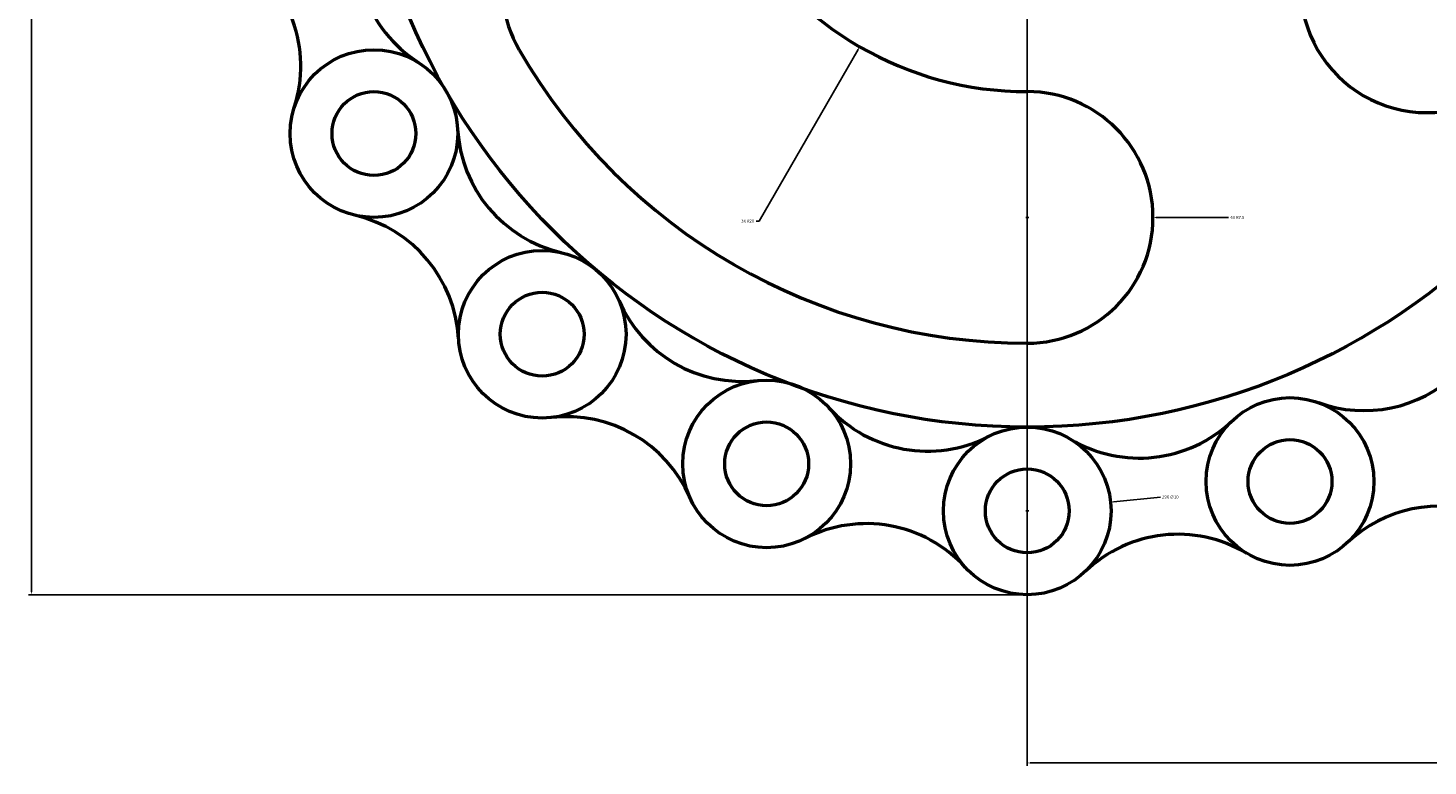
# Model space of a CAD drawing. Units: inches. Extents: x 413 to 622, y 326 to 447.
# Tile 1 of 15: x 413 to 497, y 326 to 370. Entities that reach past the tile are written whole.
import ezdxf

# ---------------------------------------------------------------- set-up
doc = ezdxf.new("R2010")
doc.units = ezdxf.units.IN
doc.header["$MEASUREMENT"] = 0
doc.layers.add('M-DIMS', color=2, linetype='Continuous', lineweight=18)
doc.layers.add('M-OUTL', color=7, linetype='Continuous', lineweight=50)
doc.styles.get("Standard").update_dxf_attribs({"font": 'arial.ttf'})
doc.dimstyles.get("Standard").update_dxf_attribs({"dimtxt": 0.18, "dimasz": 0.18, "dimexe": 0.18, "dimexo": 0.0625, "dimgap": 0.09, "dimtad": 0, "dimtih": 1, "dimtoh": 1, "dimdec": 4, "dimzin": 0, "dimdsep": 46, "dimtxsty": 'Standard', "dimcen": 0.09, "dimadec": 0, "dimazin": 0, "dimtfac": 1, "dimtdec": 4, "dimtofl": 0, "dimtmove": 0, "dimatfit": 3, "dimfxl": 1, "dimtolj": 1, "dimtzin": 0, "dimarcsym": 0})

# ---------------------------------------------------------------- blocks, each defined once
blk = doc.blocks.new('CHAIN-ROLLER-PIN')
for radius in [5, 2.5]:
    blk.add_circle((5, 5), radius)
blk = doc.blocks.new('SPROCKET-WEB-SLOT')
for centre, radius, start, end in [((7.501, 21.25), 7.5, 30, 210), ((31.317, 35), 20, 210, 270), ((31.317, 35), 35, 210, 270), ((31.317, 7.5), 7.5, 270, 90)]:
    blk.add_arc(centre, radius, start, end)
blk = doc.blocks.new('CHAIN-LINK-WAIST-P15_769')
for centre, start, end in [((6.414, 14.762), 226.27868, 300.95511), ((4.115, -5.782), 46.27868, 120.95511)]:
    blk.add_arc(centre, 8, start, end)
blk = doc.blocks.new('CHAIN-LINK-WAIST-P13_603')
for centre, start, end in [((7.205, 15.87), 226.77186, 289.86266), ((2.718, -5.829), 46.77186, 109.86266)]:
    blk.add_arc(centre, 8, start, end)
blk = doc.blocks.new('*D10')
at = {"layer": 'Defpoints', "color": 0, "transparency": 16777216}
for p in [(413.283, 436.392), (472.684, 436.392), (472.684, 336.392)]:
    blk.add_point(p, dxfattribs=at)
at = {"layer": 'M-DIMS', "color": 0, "lineweight": -2, "transparency": 16777216}
for p, q in [((472.621, 436.392), (413.103, 436.392)), ((413.283, 436.212), (413.283, 386.573)), ((413.283, 336.572), (413.283, 386.21)), ((472.621, 336.392), (413.103, 336.392))]:
    blk.add_line(p, q, dxfattribs=at)
at = {"layer": 'M-DIMS', "color": 0, "transparency": 16777216}
for points in [[(413.253, 436.212), (413.313, 436.212), (413.283, 436.392)], [(413.253, 336.572), (413.313, 336.572), (413.283, 336.392)]]:
    blk.add_solid(points, dxfattribs=at)
at = {"layer": 'M-DIMS', "color": 0, "transparency": 16777216, "insert": (413.283, 386.392), "char_height": 0.18, "attachment_point": 5}
blk.add_mtext('\\A1;100', dxfattribs=at)
blk = doc.blocks.new('*D12')
at = {"layer": 'Defpoints', "color": 0, "transparency": 16777216}
for p in [(472.684, 386.392), (592.684, 386.392), (592.684, 326.361)]:
    blk.add_point(p, dxfattribs=at)
at = {"layer": 'M-DIMS', "color": 0, "lineweight": -2, "transparency": 16777216}
for p, q in [((472.684, 386.329), (472.684, 326.181)), ((592.684, 386.329), (592.684, 326.181)), ((472.864, 326.361), (532.404, 326.361)), ((592.504, 326.361), (532.964, 326.361))]:
    blk.add_line(p, q, dxfattribs=at)
at = {"layer": 'M-DIMS', "color": 0, "transparency": 16777216}
for points in [[(472.864, 326.391), (472.864, 326.331), (472.684, 326.361)], [(592.504, 326.391), (592.504, 326.331), (592.684, 326.361)]]:
    blk.add_solid(points, dxfattribs=at)
at = {"layer": 'M-DIMS', "color": 0, "transparency": 16777216, "insert": (532.684, 326.361), "char_height": 0.18, "attachment_point": 5}
blk.add_mtext('\\A1;120', dxfattribs=at)
blk = doc.blocks.new('*D29')
at = {"layer": 'Defpoints', "color": 0, "transparency": 16777216}
for p in [(472.684, 386.392), (462.684, 369.071)]:
    blk.add_point(p, dxfattribs=at)
at = {"layer": 'M-DIMS', "color": 0, "lineweight": -2, "transparency": 16777216}
for p, q in [((472.594, 386.392), (472.774, 386.392)), ((472.684, 386.302), (472.684, 386.482)), ((456.684, 358.678), (462.594, 368.915)), ((456.504, 358.678), (456.684, 358.678))]:
    blk.add_line(p, q, dxfattribs=at)
at = {"layer": 'M-DIMS', "color": 0, "transparency": 16777216}
blk.add_solid([(462.568, 368.93), (462.62, 368.9), (462.684, 369.071)], dxfattribs=at)
at = {"layer": 'M-DIMS', "color": 0, "transparency": 16777216, "insert": (456.006, 358.678), "char_height": 0.18, "attachment_point": 5}
blk.add_mtext('\\A1;3X R20', dxfattribs=at)
blk = doc.blocks.new('*D30')
at = {"layer": 'Defpoints', "color": 0, "transparency": 16777216}
for p in [(472.684, 358.892), (480.184, 358.892)]:
    blk.add_point(p, dxfattribs=at)
at = {"layer": 'M-DIMS', "color": 0, "lineweight": -2, "transparency": 16777216}
for p, q in [((472.594, 358.892), (472.774, 358.892)), ((472.684, 358.802), (472.684, 358.982)), ((484.684, 358.892), (480.364, 358.892))]:
    blk.add_line(p, q, dxfattribs=at)
at = {"layer": 'M-DIMS', "color": 0, "transparency": 16777216}
blk.add_solid([(480.364, 358.922), (480.364, 358.862), (480.184, 358.892)], dxfattribs=at)
at = {"layer": 'M-DIMS', "color": 0, "transparency": 16777216, "insert": (485.218, 358.892), "char_height": 0.18, "attachment_point": 5}
blk.add_mtext('\\A1;6X R7.5', dxfattribs=at)
blk = doc.blocks.new('*D31')
at = {"layer": 'Defpoints', "color": 0, "transparency": 16777216}
for p in [(477.657, 341.91), (467.711, 340.873)]:
    blk.add_point(p, dxfattribs=at)
at = {"layer": 'M-DIMS', "color": 0, "lineweight": -2, "transparency": 16777216}
for p, q in [((480.641, 342.221), (477.836, 341.928)), ((472.594, 341.392), (472.774, 341.392)), ((472.684, 341.302), (472.684, 341.482))]:
    blk.add_line(p, q, dxfattribs=at)
at = {"layer": 'M-DIMS', "color": 0, "transparency": 16777216}
blk.add_solid([(477.833, 341.958), (477.839, 341.898), (477.657, 341.91)], dxfattribs=at)
at = {"layer": 'M-DIMS', "color": 0, "transparency": 16777216, "insert": (481.217, 342.221), "char_height": 0.18, "attachment_point": 5}
blk.add_mtext('\\A1;29X ∅10', dxfattribs=at)

msp = doc.modelspace()

# ---------------------------------------------------------------- linework, layer by layer
at = {"layer": 'M-OUTL'}
msp.add_circle((472.6836, 386.3915), 40, dxfattribs=at)
for centre, start, end in [((440.6768, 374.8687), 161.991387, 237.607516), ((421.3493, 367.9106), 341.991387, 57.607516), ((446.6938, 364.5884), 183.072945, 256.914229), ((430.7691, 351.2291), 3.072945, 76.914229), ((455.6707, 357.1132), 203.516756, 276.483244), ((466.7446, 352.9556), 222.360142, 297.183854), ((445.2183, 339.0091), 23.516756, 96.483244), ((463.0776, 332.6323), 42.360142, 117.183854)]:
    msp.add_arc(centre, 8, start, end, dxfattribs=at)

# ---------------------------------------------------------------- block references
for name, p, rotation in [('SPROCKET-WEB-SLOT', (518.6523, 376.7703), 119.9999999999996), ('CHAIN-LINK-WAIST-P13_603', (492.4518, 337.9457), 23.36547829356988), ('CHAIN-LINK-WAIST-P15_769', (484.6616, 347.8103), 192.76620889149)]:
    msp.add_blockref(name, p, dxfattribs=dict(at, rotation=rotation))
for name, p in [('SPROCKET-WEB-SLOT', (441.367, 351.392)), ('CHAIN-ROLLER-PIN', (428.7129, 358.892)), ('CHAIN-ROLLER-PIN', (438.7508, 346.9265)), ('CHAIN-ROLLER-PIN', (452.139, 339.1968)), ('CHAIN-ROLLER-PIN', (483.3557, 338.1452)), ('CHAIN-ROLLER-PIN', (467.684, 336.392))]:
    msp.add_blockref(name, p, dxfattribs=at)

# ---------------------------------------------------------------- dimensions: what is measured, and where the dimension line sits
at = {"layer": 'M-DIMS'}
dim = msp.add_linear_dim(base=(413.2831, 436.3915), p1=(472.6836, 336.3915), p2=(472.6836, 436.3915), angle=90, dimstyle='Standard', override={"dimdec": 0, "dimlfac": 1, "dimrnd": 0, "dimzin": 0, "dimdsep": 46, "dimlunit": 2}, dxfattribs=at)
dim.commit()
dim.dimension.update_dxf_attribs({"geometry": '*D10', "text_midpoint": (413.2831, 386.3915)})
for center, mpoint, text, override, picture, middle in [((472.6836, 386.3915), (462.6839, 369.0708), '3X <>', {"dimdec": 0, "dimlfac": 1, "dimrnd": 0, "dimzin": 0, "dimdsep": 46, "dimlunit": 2}, '*D29', (456.006, 358.6784)), ((472.6836, 358.8915), (480.1836, 358.892), '6X <>', {"dimdec": 1, "dimlfac": 1, "dimrnd": 0, "dimzin": 0, "dimdsep": 46, "dimlunit": 2}, '*D30', (484.6836, 358.8923))]:
    dim = msp.add_radius_dim(center=center, mpoint=mpoint, text=text, dimstyle='Standard', override=override, dxfattribs=at)
    dim.commit()
    dim.dimension.update_dxf_attribs({"geometry": picture, "text_midpoint": middle, "dimtype": 164})
dim = msp.add_linear_dim(base=(592.6836, 326.361), p1=(472.6836, 386.3915), p2=(592.6836, 386.3915), dimstyle='Standard', override={"dimdec": 0, "dimlfac": 1, "dimrnd": 0, "dimzin": 0, "dimdsep": 46, "dimlunit": 2}, dxfattribs=at)
dim.commit()
dim.dimension.update_dxf_attribs({"geometry": '*D12', "text_midpoint": (532.6836, 326.361)})
dim = msp.add_diameter_dim_2p(p1=(467.7105, 340.8734), p2=(477.6567, 341.9096), text='29X <>', dimstyle='Standard', override={"dimdec": 0, "dimlfac": 1, "dimrnd": 0, "dimzin": 0, "dimdsep": 46, "dimlunit": 2}, dxfattribs=at)
dim.commit()
dim.dimension.update_dxf_attribs({"geometry": '*D31', "text_midpoint": (480.6405, 342.2205), "dimtype": 163})

doc.saveas('drawing.dxf')
